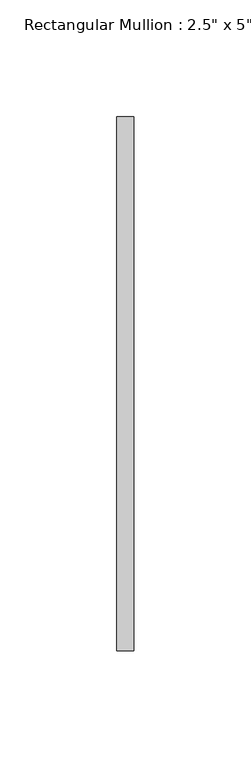
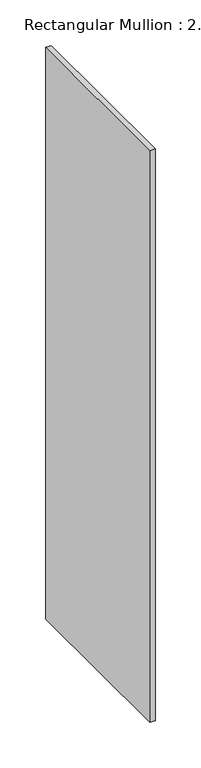
"""IFC4 building model written with IfcOpenShell, lengths in millimetres: member geometry."""

from ifc_helpers import new_model, si_unit, frame, origin, place, context, project, spatial, polyline, outline, extrude, source, transform, mapped, element, save


def member_091456ab(model_context):
    return source(origin(), model_context, "Body", "SweptSolid", [
        extrude(outline(polyline([(3.6195, 114.3), (3.6195, -114.3), (-3.6195, -114.3), (-3.6195, 114.3), (3.6195, 114.3)])), frame((0.0, 0.0, -767.0165), z_axis=(0.0, 0.0, 1.0), x_axis=(1.0, 0.0, 0.0)), (0.0, 0.0, 1.0), 767.0165),
    ])


if __name__ == "__main__":
    model = new_model("IFC4")
    model_context = context("Model", 3, world=origin())
    ifc_project = project(units=[si_unit("LENGTHUNIT", "METRE", prefix="MILLI")], contexts=[model_context])
    site = spatial("IfcSite", under=ifc_project)
    building = spatial("IfcBuilding", under=site)
    placement = place(None, origin())
    member_shape = member_091456ab(model_context)
    element("IfcMember", 1, ObjectType="Rectangular Mullion : 2.5\" x 5\" rectangular", at=placement, inside=building, context=model_context, shape_type="MappedRepresentation", body=[
        mapped(member_shape, transform((0.0, 0.0, 0.0), x_axis=(1.0, 0.0, 0.0), y_axis=(0.0, 1.0, 0.0), z_axis=(0.0, 0.0, 1.0))),
    ])
    save(model, "model.ifc")

# Revit data of these elements
# Type "Rectangular Mullion : 2.5\" x 5\" rectangular"
#   built-in parameter 1007304 = 0.75 (stored number, unit not read)
#   built-in parameter 1007301 = 0.011875 (stored number, unit not read)
#   built-in parameter 1007300 = 0.011875 (stored number, unit not read)
# Element 1 (IfcMember, "Rectangular Mullion : 2.5\" x 5\" rectangular")
#   Materials on its faces: "WINDOW GLASS MATERIAL"
# Materials
#   "WINDOW GLASS MATERIAL": class "Generic", colour RGB 120 120 120, transparency 0, Cost = 0
